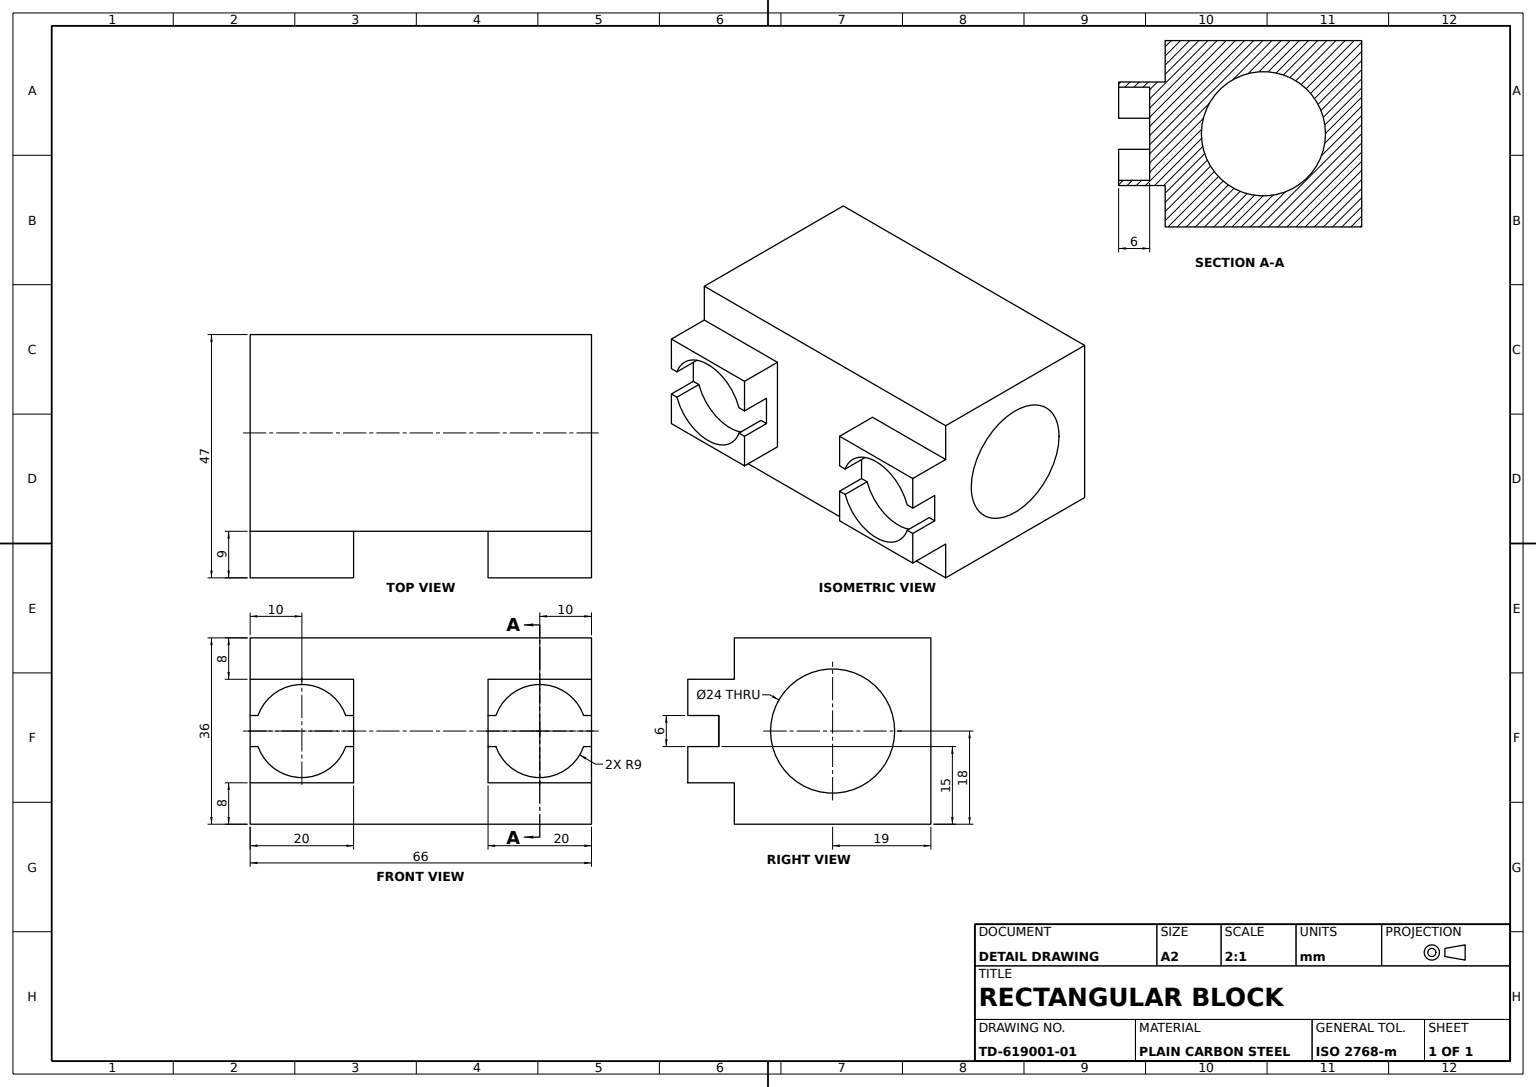
SolidWorks part; units mm, degrees
material "Plain Carbon Steel"
ref_plane "Front Plane" through (0, 0, 0) normal (0, 0, 1) x (1, 0, 0)
ref_plane "Top Plane" through (0, 0, 0) normal (0, 1, 0) x (1, 0, 0)
ref_plane "Right Plane" through (0, 0, 0) normal (1, 0, 0) x (0, 0, -1)
sketch "Main Block Profile" plane through (0, 0, 0) normal (1, 0, 0) x (0, 0, -1)
  line L1 (-33, 18) -> (33, 18)
  line L2 (-33, 18) -> (-33, -18)
  line L3 (-33, -18) -> (33, -18)
  line L4 (33, 18) -> (33, -18)
  line L5 (-33, 18) -> (33, -18) construction
  line L6 (-33, -18) -> (33, 18) construction
  point P0 (0, 0)
  dimension "D1" = 66
  dimension "D2" = 36
extrude "Main Block 66x36x38" add sketch "Main Block Profile" along normal blind 38
sketch "Clamp Bosses Profile" plane through (38, 0, 0) normal (1, 0, 0) x (0, 0, -1)
  line L0 (-33, 10) -> (-13, 10)
  line L1 (33, 10) -> (13, 10)
  line L6 (-33, 18) -> (-33, -18) construction
  line L7 (-13, 10) -> (-13, -10)
  line L8 (-13, -10) -> (-33, -10)
  line L9 (-33, -10) -> (-33, 10)
  line L10 (33, -18) -> (33, 18) construction
  line L11 (13, 10) -> (13, -10)
  line L12 (13, -10) -> (33, -10)
  line L13 (33, -10) -> (33, 10)
  dimension "D1" = 8
  dimension "D2" = 8
  dimension "D3" = 20
  dimension "D4" = 20
  dimension "D5" = 8
extrude "Clamp Bosses" add sketch "Clamp Bosses Profile" along normal blind 9
sketch "Saddle Cut Ø18 A Profile" plane through (47, 0, 0) normal (1, 0, 0) x (0, 0, -1)
  line L0 (-33, 10) -> (-33, -10) construction
  circle A0 centre (-23, 0) radius 9
  dimension "D1" = 18
  dimension "D2" = 10
extrude "Saddle Cut Ø18 A" cut sketch "Saddle Cut Ø18 A Profile" against normal blind 6
sketch "Notch A Profile" plane through (0, 0, 33) normal (0, 0, 1) x (1, 0, 0)
  line L0 (47, 0) -> (41, 0) construction
  line L1 (47, 10) -> (47, -10) construction
  line L2 (41, 0) -> (41, 3)
  line L3 (41, 3) -> (47, 3)
  line L4 (41, 0) -> (41, -3)
  line L5 (41, -3) -> (47, -3)
  dimension "D1" = 3
  dimension "D2" = 3
  dimension "D3" = 6
extrude "Notch A 3x3" cut sketch "Notch A Profile" against normal blind 6 and the other way through all
sketch "Notch B Profile" plane through (0, 0, 13) normal (0, 0, -1) x (-1, 0, 0)
  line L0 (-47, 0) -> (-41, 0) construction
  line L1 (-47, -10) -> (-47, 10) construction
  line L2 (-41, 0) -> (-41, 3)
  line L3 (-41, 3) -> (-47, 3)
  line L4 (-47, 3) -> (-47, -3)
  line L5 (-47, -3) -> (-41, -3)
  line L6 (-41, -3) -> (-41, 0)
  dimension "D1" = 3
  dimension "D2" = 3
  dimension "D3" = 6
extrude "Notch B 3x3" cut sketch "Notch B Profile" against normal blind 6
sketch "Saddle Cut Ø18 B Profile" plane through (47, 0, 0) normal (1, 0, 0) x (0, 0, -1)
  line L0 (13, 10) -> (13, -10) construction
  circle A0 centre (23, 0) radius 9
  dimension "D1" = 18
  dimension "D2" = 10
extrude "Saddle Cut Ø18 B" cut sketch "Saddle Cut Ø18 B Profile" against normal blind 6
sketch "Notch C Profile" plane through (0, 0, -33) normal (0, 0, -1) x (-1, 0, 0)
  line L0 (-47, 0) -> (-41, 0) construction
  line L1 (-47, -10) -> (-47, 10) construction
  line L2 (-41, 0) -> (-41, 3)
  line L3 (-41, 3) -> (-47, 3)
  line L4 (-47, 3) -> (-47, -3)
  line L5 (-47, -3) -> (-41, -3)
  line L6 (-41, -3) -> (-41, 0)
  dimension "D1" = 3
  dimension "D2" = 3
  dimension "D3" = 6
extrude "Notch C 3x3" cut sketch "Notch C Profile" against normal blind 6
sketch "Notch D Profile" plane through (0, 0, -13) normal (0, 0, 1) x (1, 0, 0)
  line L0 (47, 3) -> (41, 3)
  line L1 (47, 10) -> (47, -10) construction
  line L2 (47, 10) -> (47, 3) construction
  line L3 (41, 3) -> (41, -3)
  line L4 (41, -3) -> (47, -3)
  line L5 (47, -3) -> (47, 3)
extrude "Notch D" cut sketch "Notch D Profile" against normal blind 6
sketch "End Bore Ø24 Profile" plane through (0, 0, 33) normal (0, 0, 1) x (1, 0, 0)
  line L0 (19, -18) -> (19, 18) construction
  line L1 (38, -18) -> (0, -18) construction
  line L2 (38, 18) -> (0, 18) construction
  circle A0 centre (19, 0) radius 12
  dimension "D1" = 24
extrude "End Bore Ø24" cut sketch "End Bore Ø24 Profile" against normal through all
